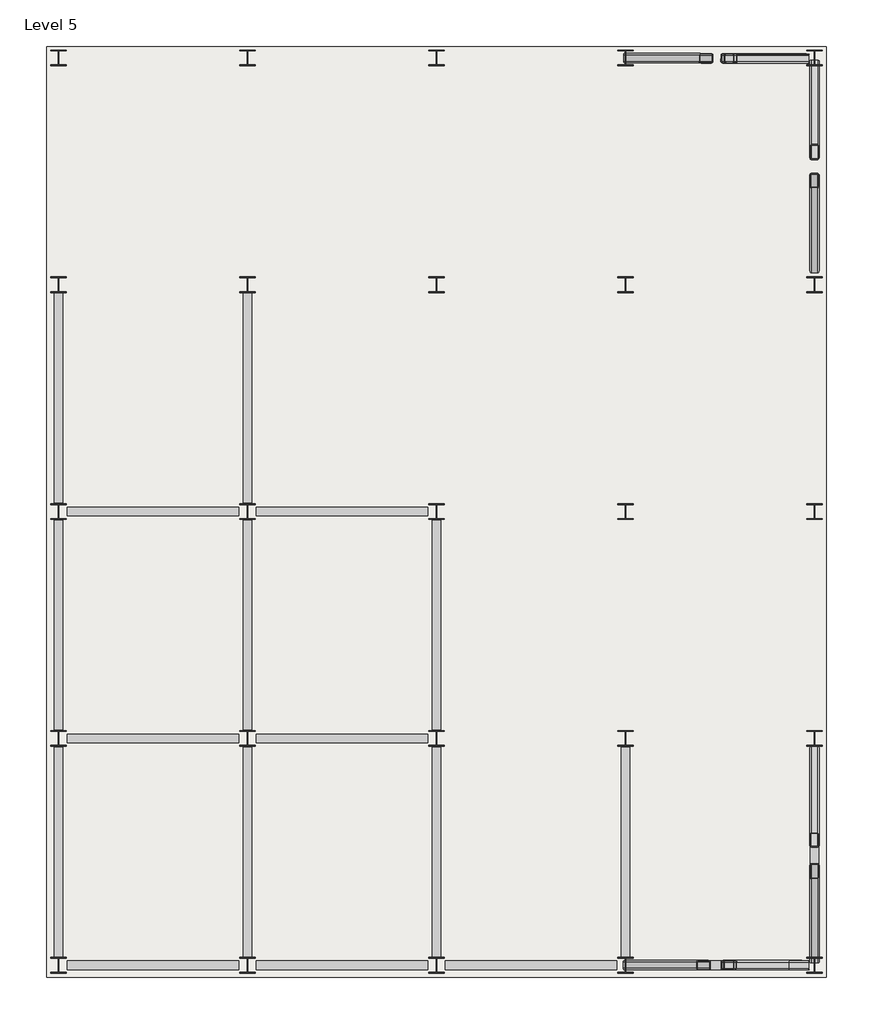
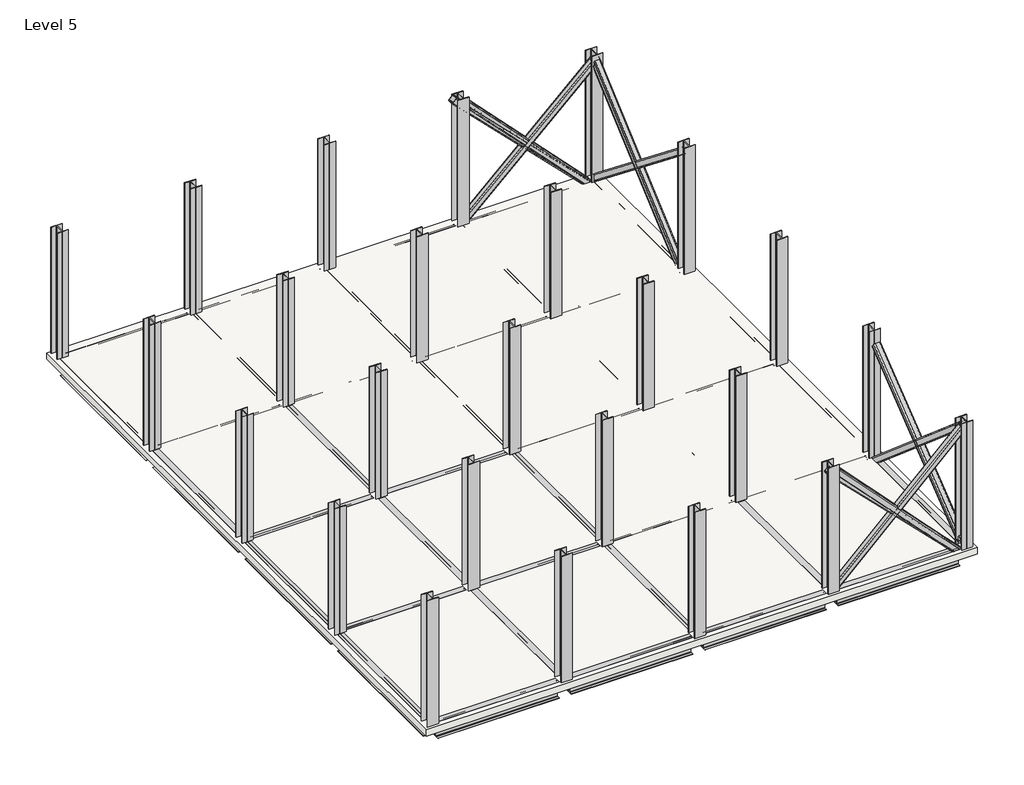
# One storey: 40 beams, 25 columns, 10 members, 1 slab.
"""IFC4 building model written with IfcOpenShell, lengths in millimetres."""

from ifc_helpers import new_model, si_unit, frame, origin, place, context, project, spatial, polyline, outline, extrude, transform, mapped, element, save
from components import w_shapes_w16x26_71b85d0e, w_shapes_w16x26_5730d789, w_shapes_column_w10x49_51893fb5, hss_square_hss6x6x1_2_008024fe, hss_square_hss6x6x1_2_53b34d95, hss_square_hss6x6x1_2_5f011b37, hss_square_hss6x6x1_2_b9926e2d, hss_square_hss6x6x1_2_d64262a5, hss_square_hss6x6x1_2_e6555cf9, hss_square_hss6x6x1_2_f7a49a43, hss_square_hss6x6x1_2_c82ee425, hss_square_hss6x6x1_2_10b7330d, hss_square_hss6x6x1_2_f3b36863

model = new_model("IFC4")

# Units and contexts
model_context = context("Model", 3, world=origin())
ifc_project = project(units=[si_unit("LENGTHUNIT", "METRE", prefix="MILLI")], contexts=[model_context])

# Site, building, storey
site = spatial("IfcSite", under=ifc_project)
building = spatial("IfcBuilding", under=site)
storey = spatial("IfcBuildingStorey", under=building, Name="Level 5", Elevation=12192.0)

# Beams
placement = place(None, origin())
w_shapes_w16x26_shape = w_shapes_w16x26_71b85d0e(model_context)
element("IfcBeam", 1, ObjectType="W Shapes : W16X26", at=placement, inside=storey, context=model_context, shape_type="MappedRepresentation", body=[
    mapped(w_shapes_w16x26_shape, transform((-5883.5186598, -2213.7239423, 11992.61), x_axis=(1.0, 0.0, 0.0), y_axis=(0.0, 1.0, 0.0), z_axis=(0.0, 0.0, 1.0))),
])
element("IfcBeam", 2, ObjectType="W Shapes : W16X26", at=placement, inside=storey, context=model_context, shape_type="MappedRepresentation", body=[
    mapped(w_shapes_w16x26_shape, transform((-2835.5186598, -2213.7239423, 11992.61), x_axis=(1.0, 0.0, 0.0), y_axis=(0.0, 1.0, 0.0), z_axis=(0.0, 0.0, 1.0))),
])
element("IfcBeam", 3, ObjectType="W Shapes : W16X26", at=placement, inside=storey, context=model_context, shape_type="MappedRepresentation", body=[
    mapped(w_shapes_w16x26_shape, transform((212.4813402, -2213.7239423, 11992.61), x_axis=(1.0, 0.0, 0.0), y_axis=(0.0, 1.0, 0.0), z_axis=(0.0, 0.0, 1.0))),
])
element("IfcBeam", 4, ObjectType="W Shapes : W16X26", at=placement, inside=storey, context=model_context, shape_type="MappedRepresentation", body=[
    mapped(w_shapes_w16x26_shape, transform((3260.4813402, -2213.7239423, 11992.61), x_axis=(1.0, 0.0, 0.0), y_axis=(0.0, 1.0, 0.0), z_axis=(0.0, 0.0, 1.0))),
])
element("IfcBeam", 5, ObjectType="W Shapes : W16X26", at=placement, inside=storey, context=model_context, shape_type="MappedRepresentation", body=[
    mapped(w_shapes_w16x26_shape, transform((-5883.5186598, 1443.8760577, 11992.61), x_axis=(1.0, 0.0, 0.0), y_axis=(0.0, 1.0, 0.0), z_axis=(0.0, 0.0, 1.0))),
])
element("IfcBeam", 6, ObjectType="W Shapes : W16X26", at=placement, inside=storey, context=model_context, shape_type="MappedRepresentation", body=[
    mapped(w_shapes_w16x26_shape, transform((-2835.5186598, 1443.8760577, 11992.61), x_axis=(1.0, 0.0, 0.0), y_axis=(0.0, 1.0, 0.0), z_axis=(0.0, 0.0, 1.0))),
])
element("IfcBeam", 7, ObjectType="W Shapes : W16X26", at=placement, inside=storey, context=model_context, shape_type="MappedRepresentation", body=[
    mapped(w_shapes_w16x26_shape, transform((212.4813402, 1443.8760577, 11992.61), x_axis=(1.0, 0.0, 0.0), y_axis=(0.0, 1.0, 0.0), z_axis=(0.0, 0.0, 1.0))),
])
element("IfcBeam", 8, ObjectType="W Shapes : W16X26", at=placement, inside=storey, context=model_context, shape_type="MappedRepresentation", body=[
    mapped(w_shapes_w16x26_shape, transform((3260.4813402, 1443.8760577, 11992.61), x_axis=(1.0, 0.0, 0.0), y_axis=(0.0, 1.0, 0.0), z_axis=(0.0, 0.0, 1.0))),
])
element("IfcBeam", 9, ObjectType="W Shapes : W16X26", at=placement, inside=storey, context=model_context, shape_type="MappedRepresentation", body=[
    mapped(w_shapes_w16x26_shape, transform((-5883.5186598, 5101.4760577, 11992.61), x_axis=(1.0, 0.0, 0.0), y_axis=(0.0, 1.0, 0.0), z_axis=(0.0, 0.0, 1.0))),
])
element("IfcBeam", 10, ObjectType="W Shapes : W16X26", at=placement, inside=storey, context=model_context, shape_type="MappedRepresentation", body=[
    mapped(w_shapes_w16x26_shape, transform((-2835.5186598, 5101.4760577, 11992.61), x_axis=(1.0, 0.0, 0.0), y_axis=(0.0, 1.0, 0.0), z_axis=(0.0, 0.0, 1.0))),
])
element("IfcBeam", 11, ObjectType="W Shapes : W16X26", at=placement, inside=storey, context=model_context, shape_type="MappedRepresentation", body=[
    mapped(w_shapes_w16x26_shape, transform((212.4813402, 5101.4760577, 11992.61), x_axis=(1.0, 0.0, 0.0), y_axis=(0.0, 1.0, 0.0), z_axis=(0.0, 0.0, 1.0))),
])
element("IfcBeam", 12, ObjectType="W Shapes : W16X26", at=placement, inside=storey, context=model_context, shape_type="MappedRepresentation", body=[
    mapped(w_shapes_w16x26_shape, transform((3260.4813402, 5101.4760577, 11992.61), x_axis=(1.0, 0.0, 0.0), y_axis=(0.0, 1.0, 0.0), z_axis=(0.0, 0.0, 1.0))),
])
element("IfcBeam", 13, ObjectType="W Shapes : W16X26", at=placement, inside=storey, context=model_context, shape_type="MappedRepresentation", body=[
    mapped(w_shapes_w16x26_shape, transform((-5883.5186598, 8759.0760577, 11992.61), x_axis=(1.0, 0.0, 0.0), y_axis=(0.0, 1.0, 0.0), z_axis=(0.0, 0.0, 1.0))),
])
element("IfcBeam", 14, ObjectType="W Shapes : W16X26", at=placement, inside=storey, context=model_context, shape_type="MappedRepresentation", body=[
    mapped(w_shapes_w16x26_shape, transform((-2835.5186598, 8759.0760577, 11992.61), x_axis=(1.0, 0.0, 0.0), y_axis=(0.0, 1.0, 0.0), z_axis=(0.0, 0.0, 1.0))),
])
element("IfcBeam", 15, ObjectType="W Shapes : W16X26", at=placement, inside=storey, context=model_context, shape_type="MappedRepresentation", body=[
    mapped(w_shapes_w16x26_shape, transform((212.4813402, 8759.0760577, 11992.61), x_axis=(1.0, 0.0, 0.0), y_axis=(0.0, 1.0, 0.0), z_axis=(0.0, 0.0, 1.0))),
])
element("IfcBeam", 16, ObjectType="W Shapes : W16X26", at=placement, inside=storey, context=model_context, shape_type="MappedRepresentation", body=[
    mapped(w_shapes_w16x26_shape, transform((3260.4813402, 8759.0760577, 11992.61), x_axis=(1.0, 0.0, 0.0), y_axis=(0.0, 1.0, 0.0), z_axis=(0.0, 0.0, 1.0))),
])
element("IfcBeam", 17, ObjectType="W Shapes : W16X26", at=placement, inside=storey, context=model_context, shape_type="MappedRepresentation", body=[
    mapped(w_shapes_w16x26_shape, transform((-5883.5186598, 12416.6760577, 11992.61), x_axis=(1.0, 0.0, 0.0), y_axis=(0.0, 1.0, 0.0), z_axis=(0.0, 0.0, 1.0))),
])
element("IfcBeam", 18, ObjectType="W Shapes : W16X26", at=placement, inside=storey, context=model_context, shape_type="MappedRepresentation", body=[
    mapped(w_shapes_w16x26_shape, transform((-2835.5186598, 12416.6760577, 11992.61), x_axis=(1.0, 0.0, 0.0), y_axis=(0.0, 1.0, 0.0), z_axis=(0.0, 0.0, 1.0))),
])
element("IfcBeam", 19, ObjectType="W Shapes : W16X26", at=placement, inside=storey, context=model_context, shape_type="MappedRepresentation", body=[
    mapped(w_shapes_w16x26_shape, transform((212.4813402, 12416.6760577, 11992.61), x_axis=(1.0, 0.0, 0.0), y_axis=(0.0, 1.0, 0.0), z_axis=(0.0, 0.0, 1.0))),
])
element("IfcBeam", 20, ObjectType="W Shapes : W16X26", at=placement, inside=storey, context=model_context, shape_type="MappedRepresentation", body=[
    mapped(w_shapes_w16x26_shape, transform((3260.4813402, 12416.6760577, 11992.61), x_axis=(1.0, 0.0, 0.0), y_axis=(0.0, 1.0, 0.0), z_axis=(0.0, 0.0, 1.0))),
])
w_shapes_w16x26_2_shape = w_shapes_w16x26_5730d789(model_context)
element("IfcBeam", 21, ObjectType="W Shapes : W16X26", at=placement, inside=storey, context=model_context, shape_type="MappedRepresentation", body=[
    mapped(w_shapes_w16x26_2_shape, transform((4784.4813402, 10587.8760577, 11992.61), x_axis=(0.0, -1.0, 0.0), y_axis=(1.0, 0.0, 0.0), z_axis=(0.0, 0.0, 1.0))),
])
element("IfcBeam", 22, ObjectType="W Shapes : W16X26", at=placement, inside=storey, context=model_context, shape_type="MappedRepresentation", body=[
    mapped(w_shapes_w16x26_2_shape, transform((4784.4813402, 6930.2760577, 11992.61), x_axis=(0.0, -1.0, 0.0), y_axis=(1.0, 0.0, 0.0), z_axis=(0.0, 0.0, 1.0))),
])
element("IfcBeam", 23, ObjectType="W Shapes : W16X26", at=placement, inside=storey, context=model_context, shape_type="MappedRepresentation", body=[
    mapped(w_shapes_w16x26_2_shape, transform((4784.4813402, 3272.6760577, 11992.61), x_axis=(0.0, -1.0, 0.0), y_axis=(1.0, 0.0, 0.0), z_axis=(0.0, 0.0, 1.0))),
])
element("IfcBeam", 24, ObjectType="W Shapes : W16X26", at=placement, inside=storey, context=model_context, shape_type="MappedRepresentation", body=[
    mapped(w_shapes_w16x26_2_shape, transform((4784.4813402, -384.9239423, 11992.61), x_axis=(0.0, -1.0, 0.0), y_axis=(1.0, 0.0, 0.0), z_axis=(0.0, 0.0, 1.0))),
])
element("IfcBeam", 25, ObjectType="W Shapes : W16X26", at=placement, inside=storey, context=model_context, shape_type="MappedRepresentation", body=[
    mapped(w_shapes_w16x26_2_shape, transform((1736.4813402, 10587.8760577, 11992.61), x_axis=(0.0, -1.0, 0.0), y_axis=(1.0, 0.0, 0.0), z_axis=(0.0, 0.0, 1.0))),
])
element("IfcBeam", 26, ObjectType="W Shapes : W16X26", at=placement, inside=storey, context=model_context, shape_type="MappedRepresentation", body=[
    mapped(w_shapes_w16x26_2_shape, transform((1736.4813402, 6930.2760577, 11992.61), x_axis=(0.0, -1.0, 0.0), y_axis=(1.0, 0.0, 0.0), z_axis=(0.0, 0.0, 1.0))),
])
element("IfcBeam", 27, ObjectType="W Shapes : W16X26", at=placement, inside=storey, context=model_context, shape_type="MappedRepresentation", body=[
    mapped(w_shapes_w16x26_2_shape, transform((1736.4813402, 3272.6760577, 11992.61), x_axis=(0.0, -1.0, 0.0), y_axis=(1.0, 0.0, 0.0), z_axis=(0.0, 0.0, 1.0))),
])
element("IfcBeam", 28, ObjectType="W Shapes : W16X26", at=placement, inside=storey, context=model_context, shape_type="MappedRepresentation", body=[
    mapped(w_shapes_w16x26_2_shape, transform((1736.4813402, -384.9239423, 11992.61), x_axis=(0.0, -1.0, 0.0), y_axis=(1.0, 0.0, 0.0), z_axis=(0.0, 0.0, 1.0))),
])
element("IfcBeam", 29, ObjectType="W Shapes : W16X26", at=placement, inside=storey, context=model_context, shape_type="MappedRepresentation", body=[
    mapped(w_shapes_w16x26_2_shape, transform((-1311.5186598, 10587.8760577, 11992.61), x_axis=(0.0, -1.0, 0.0), y_axis=(1.0, 0.0, 0.0), z_axis=(0.0, 0.0, 1.0))),
])
element("IfcBeam", 30, ObjectType="W Shapes : W16X26", at=placement, inside=storey, context=model_context, shape_type="MappedRepresentation", body=[
    mapped(w_shapes_w16x26_2_shape, transform((-1311.5186598, 6930.2760577, 11992.61), x_axis=(0.0, -1.0, 0.0), y_axis=(1.0, 0.0, 0.0), z_axis=(0.0, 0.0, 1.0))),
])
element("IfcBeam", 31, ObjectType="W Shapes : W16X26", at=placement, inside=storey, context=model_context, shape_type="MappedRepresentation", body=[
    mapped(w_shapes_w16x26_2_shape, transform((-1311.5186598, 3272.6760577, 11992.61), x_axis=(0.0, -1.0, 0.0), y_axis=(1.0, 0.0, 0.0), z_axis=(0.0, 0.0, 1.0))),
])
element("IfcBeam", 32, ObjectType="W Shapes : W16X26", at=placement, inside=storey, context=model_context, shape_type="MappedRepresentation", body=[
    mapped(w_shapes_w16x26_2_shape, transform((-1311.5186598, -384.9239423, 11992.61), x_axis=(0.0, -1.0, 0.0), y_axis=(1.0, 0.0, 0.0), z_axis=(0.0, 0.0, 1.0))),
])
element("IfcBeam", 33, ObjectType="W Shapes : W16X26", at=placement, inside=storey, context=model_context, shape_type="MappedRepresentation", body=[
    mapped(w_shapes_w16x26_2_shape, transform((-4359.5186598, 10587.8760577, 11992.61), x_axis=(0.0, -1.0, 0.0), y_axis=(1.0, 0.0, 0.0), z_axis=(0.0, 0.0, 1.0))),
])
element("IfcBeam", 34, ObjectType="W Shapes : W16X26", at=placement, inside=storey, context=model_context, shape_type="MappedRepresentation", body=[
    mapped(w_shapes_w16x26_2_shape, transform((-4359.5186598, 6930.2760577, 11992.61), x_axis=(0.0, -1.0, 0.0), y_axis=(1.0, 0.0, 0.0), z_axis=(0.0, 0.0, 1.0))),
])
element("IfcBeam", 35, ObjectType="W Shapes : W16X26", at=placement, inside=storey, context=model_context, shape_type="MappedRepresentation", body=[
    mapped(w_shapes_w16x26_2_shape, transform((-4359.5186598, 3272.6760577, 11992.61), x_axis=(0.0, -1.0, 0.0), y_axis=(1.0, 0.0, 0.0), z_axis=(0.0, 0.0, 1.0))),
])
element("IfcBeam", 36, ObjectType="W Shapes : W16X26", at=placement, inside=storey, context=model_context, shape_type="MappedRepresentation", body=[
    mapped(w_shapes_w16x26_2_shape, transform((-4359.5186598, -384.9239423, 11992.61), x_axis=(0.0, -1.0, 0.0), y_axis=(1.0, 0.0, 0.0), z_axis=(0.0, 0.0, 1.0))),
])
element("IfcBeam", 37, ObjectType="W Shapes : W16X26", at=placement, inside=storey, context=model_context, shape_type="MappedRepresentation", body=[
    mapped(w_shapes_w16x26_2_shape, transform((-7407.5186598, 10587.8760577, 11992.61), x_axis=(0.0, -1.0, 0.0), y_axis=(1.0, 0.0, 0.0), z_axis=(0.0, 0.0, 1.0))),
])
element("IfcBeam", 38, ObjectType="W Shapes : W16X26", at=placement, inside=storey, context=model_context, shape_type="MappedRepresentation", body=[
    mapped(w_shapes_w16x26_2_shape, transform((-7407.5186598, 6930.2760577, 11992.61), x_axis=(0.0, -1.0, 0.0), y_axis=(1.0, 0.0, 0.0), z_axis=(0.0, 0.0, 1.0))),
])
element("IfcBeam", 39, ObjectType="W Shapes : W16X26", at=placement, inside=storey, context=model_context, shape_type="MappedRepresentation", body=[
    mapped(w_shapes_w16x26_2_shape, transform((-7407.5186598, 3272.6760577, 11992.61), x_axis=(0.0, -1.0, 0.0), y_axis=(1.0, 0.0, 0.0), z_axis=(0.0, 0.0, 1.0))),
])
element("IfcBeam", 40, ObjectType="W Shapes : W16X26", at=placement, inside=storey, context=model_context, shape_type="MappedRepresentation", body=[
    mapped(w_shapes_w16x26_2_shape, transform((-7407.5186598, -384.9239423, 11992.61), x_axis=(0.0, -1.0, 0.0), y_axis=(1.0, 0.0, 0.0), z_axis=(0.0, 0.0, 1.0))),
])

# Columns
w_shapes_column_w10x49_shape = w_shapes_column_w10x49_51893fb5(model_context)
element("IfcColumn", 41, ObjectType="W Shapes-Column : W10X49", at=placement, inside=storey, context=model_context, shape_type="MappedRepresentation", body=[
    mapped(w_shapes_column_w10x49_shape, transform((4784.4813402, -2213.7239423, 0.0), x_axis=(1.0, 0.0, 0.0), y_axis=(0.0, 1.0, 0.0), z_axis=(0.0, 0.0, 1.0))),
])
element("IfcColumn", 42, ObjectType="W Shapes-Column : W10X49", at=placement, inside=storey, context=model_context, shape_type="MappedRepresentation", body=[
    mapped(w_shapes_column_w10x49_shape, transform((1736.4813402, -2213.7239423, 0.0), x_axis=(1.0, 0.0, 0.0), y_axis=(0.0, 1.0, 0.0), z_axis=(0.0, 0.0, 1.0))),
])
element("IfcColumn", 43, ObjectType="W Shapes-Column : W10X49", at=placement, inside=storey, context=model_context, shape_type="MappedRepresentation", body=[
    mapped(w_shapes_column_w10x49_shape, transform((-1311.5186598, -2213.7239423, 0.0), x_axis=(1.0, 0.0, 0.0), y_axis=(0.0, 1.0, 0.0), z_axis=(0.0, 0.0, 1.0))),
])
element("IfcColumn", 44, ObjectType="W Shapes-Column : W10X49", at=placement, inside=storey, context=model_context, shape_type="MappedRepresentation", body=[
    mapped(w_shapes_column_w10x49_shape, transform((-4359.5186598, -2213.7239423, 0.0), x_axis=(1.0, 0.0, 0.0), y_axis=(0.0, 1.0, 0.0), z_axis=(0.0, 0.0, 1.0))),
])
element("IfcColumn", 45, ObjectType="W Shapes-Column : W10X49", at=placement, inside=storey, context=model_context, shape_type="MappedRepresentation", body=[
    mapped(w_shapes_column_w10x49_shape, transform((-7407.5186598, -2213.7239423, 0.0), x_axis=(1.0, 0.0, 0.0), y_axis=(0.0, 1.0, 0.0), z_axis=(0.0, 0.0, 1.0))),
])
element("IfcColumn", 46, ObjectType="W Shapes-Column : W10X49", at=placement, inside=storey, context=model_context, shape_type="MappedRepresentation", body=[
    mapped(w_shapes_column_w10x49_shape, transform((4784.4813402, 1443.8760577, 0.0), x_axis=(1.0, 0.0, 0.0), y_axis=(0.0, 1.0, 0.0), z_axis=(0.0, 0.0, 1.0))),
])
element("IfcColumn", 47, ObjectType="W Shapes-Column : W10X49", at=placement, inside=storey, context=model_context, shape_type="MappedRepresentation", body=[
    mapped(w_shapes_column_w10x49_shape, transform((4784.4813402, 5101.4760577, 0.0), x_axis=(1.0, 0.0, 0.0), y_axis=(0.0, 1.0, 0.0), z_axis=(0.0, 0.0, 1.0))),
])
element("IfcColumn", 48, ObjectType="W Shapes-Column : W10X49", at=placement, inside=storey, context=model_context, shape_type="MappedRepresentation", body=[
    mapped(w_shapes_column_w10x49_shape, transform((4784.4813402, 8759.0760577, 0.0), x_axis=(1.0, 0.0, 0.0), y_axis=(0.0, 1.0, 0.0), z_axis=(0.0, 0.0, 1.0))),
])
element("IfcColumn", 49, ObjectType="W Shapes-Column : W10X49", at=placement, inside=storey, context=model_context, shape_type="MappedRepresentation", body=[
    mapped(w_shapes_column_w10x49_shape, transform((4784.4813402, 12416.6760577, 0.0), x_axis=(1.0, 0.0, 0.0), y_axis=(0.0, 1.0, 0.0), z_axis=(0.0, 0.0, 1.0))),
])
element("IfcColumn", 50, ObjectType="W Shapes-Column : W10X49", at=placement, inside=storey, context=model_context, shape_type="MappedRepresentation", body=[
    mapped(w_shapes_column_w10x49_shape, transform((1736.4813402, 1443.8760577, 0.0), x_axis=(1.0, 0.0, 0.0), y_axis=(0.0, 1.0, 0.0), z_axis=(0.0, 0.0, 1.0))),
])
element("IfcColumn", 51, ObjectType="W Shapes-Column : W10X49", at=placement, inside=storey, context=model_context, shape_type="MappedRepresentation", body=[
    mapped(w_shapes_column_w10x49_shape, transform((-1311.5186598, 1443.8760577, 0.0), x_axis=(1.0, 0.0, 0.0), y_axis=(0.0, 1.0, 0.0), z_axis=(0.0, 0.0, 1.0))),
])
element("IfcColumn", 52, ObjectType="W Shapes-Column : W10X49", at=placement, inside=storey, context=model_context, shape_type="MappedRepresentation", body=[
    mapped(w_shapes_column_w10x49_shape, transform((-4359.5186598, 1443.8760577, 0.0), x_axis=(1.0, 0.0, 0.0), y_axis=(0.0, 1.0, 0.0), z_axis=(0.0, 0.0, 1.0))),
])
element("IfcColumn", 53, ObjectType="W Shapes-Column : W10X49", at=placement, inside=storey, context=model_context, shape_type="MappedRepresentation", body=[
    mapped(w_shapes_column_w10x49_shape, transform((-7407.5186598, 1443.8760577, 0.0), x_axis=(1.0, 0.0, 0.0), y_axis=(0.0, 1.0, 0.0), z_axis=(0.0, 0.0, 1.0))),
])
element("IfcColumn", 54, ObjectType="W Shapes-Column : W10X49", at=placement, inside=storey, context=model_context, shape_type="MappedRepresentation", body=[
    mapped(w_shapes_column_w10x49_shape, transform((1736.4813402, 5101.4760577, 0.0), x_axis=(1.0, 0.0, 0.0), y_axis=(0.0, 1.0, 0.0), z_axis=(0.0, 0.0, 1.0))),
])
element("IfcColumn", 55, ObjectType="W Shapes-Column : W10X49", at=placement, inside=storey, context=model_context, shape_type="MappedRepresentation", body=[
    mapped(w_shapes_column_w10x49_shape, transform((-1311.5186598, 5101.4760577, 0.0), x_axis=(1.0, 0.0, 0.0), y_axis=(0.0, 1.0, 0.0), z_axis=(0.0, 0.0, 1.0))),
])
element("IfcColumn", 56, ObjectType="W Shapes-Column : W10X49", at=placement, inside=storey, context=model_context, shape_type="MappedRepresentation", body=[
    mapped(w_shapes_column_w10x49_shape, transform((-4359.5186598, 5101.4760577, 0.0), x_axis=(1.0, 0.0, 0.0), y_axis=(0.0, 1.0, 0.0), z_axis=(0.0, 0.0, 1.0))),
])
element("IfcColumn", 57, ObjectType="W Shapes-Column : W10X49", at=placement, inside=storey, context=model_context, shape_type="MappedRepresentation", body=[
    mapped(w_shapes_column_w10x49_shape, transform((-7407.5186598, 5101.4760577, 0.0), x_axis=(1.0, 0.0, 0.0), y_axis=(0.0, 1.0, 0.0), z_axis=(0.0, 0.0, 1.0))),
])
element("IfcColumn", 58, ObjectType="W Shapes-Column : W10X49", at=placement, inside=storey, context=model_context, shape_type="MappedRepresentation", body=[
    mapped(w_shapes_column_w10x49_shape, transform((1736.4813402, 8759.0760577, 0.0), x_axis=(1.0, 0.0, 0.0), y_axis=(0.0, 1.0, 0.0), z_axis=(0.0, 0.0, 1.0))),
])
element("IfcColumn", 59, ObjectType="W Shapes-Column : W10X49", at=placement, inside=storey, context=model_context, shape_type="MappedRepresentation", body=[
    mapped(w_shapes_column_w10x49_shape, transform((-1311.5186598, 8759.0760577, 0.0), x_axis=(1.0, 0.0, 0.0), y_axis=(0.0, 1.0, 0.0), z_axis=(0.0, 0.0, 1.0))),
])
element("IfcColumn", 60, ObjectType="W Shapes-Column : W10X49", at=placement, inside=storey, context=model_context, shape_type="MappedRepresentation", body=[
    mapped(w_shapes_column_w10x49_shape, transform((-4359.5186598, 8759.0760577, 0.0), x_axis=(1.0, 0.0, 0.0), y_axis=(0.0, 1.0, 0.0), z_axis=(0.0, 0.0, 1.0))),
])
element("IfcColumn", 61, ObjectType="W Shapes-Column : W10X49", at=placement, inside=storey, context=model_context, shape_type="MappedRepresentation", body=[
    mapped(w_shapes_column_w10x49_shape, transform((-7407.5186598, 8759.0760577, 0.0), x_axis=(1.0, 0.0, 0.0), y_axis=(0.0, 1.0, 0.0), z_axis=(0.0, 0.0, 1.0))),
])
element("IfcColumn", 62, ObjectType="W Shapes-Column : W10X49", at=placement, inside=storey, context=model_context, shape_type="MappedRepresentation", body=[
    mapped(w_shapes_column_w10x49_shape, transform((1736.4813402, 12416.6760577, 0.0), x_axis=(1.0, 0.0, 0.0), y_axis=(0.0, 1.0, 0.0), z_axis=(0.0, 0.0, 1.0))),
])
element("IfcColumn", 63, ObjectType="W Shapes-Column : W10X49", at=placement, inside=storey, context=model_context, shape_type="MappedRepresentation", body=[
    mapped(w_shapes_column_w10x49_shape, transform((-1311.5186598, 12416.6760577, 0.0), x_axis=(1.0, 0.0, 0.0), y_axis=(0.0, 1.0, 0.0), z_axis=(0.0, 0.0, 1.0))),
])
element("IfcColumn", 64, ObjectType="W Shapes-Column : W10X49", at=placement, inside=storey, context=model_context, shape_type="MappedRepresentation", body=[
    mapped(w_shapes_column_w10x49_shape, transform((-4359.5186598, 12416.6760577, 0.0), x_axis=(1.0, 0.0, 0.0), y_axis=(0.0, 1.0, 0.0), z_axis=(0.0, 0.0, 1.0))),
])
element("IfcColumn", 65, ObjectType="W Shapes-Column : W10X49", at=placement, inside=storey, context=model_context, shape_type="MappedRepresentation", body=[
    mapped(w_shapes_column_w10x49_shape, transform((-7407.5186598, 12416.6760577, 0.0), x_axis=(1.0, 0.0, 0.0), y_axis=(0.0, 1.0, 0.0), z_axis=(0.0, 0.0, 1.0))),
])

# Members
hss_square_hss6x6x1_2_shape = hss_square_hss6x6x1_2_008024fe(model_context)
element("IfcMember", 66, ObjectType="HSS Square : HSS6X6X1/2", at=placement, inside=storey, context=model_context, shape_type="MappedRepresentation", body=[
    mapped(hss_square_hss6x6x1_2_shape, transform((4784.4813402, 10587.8760577, 13639.8), x_axis=(0.0, 0.7840458244617616, -0.6207029443655613), y_axis=(-1.0000000000000002, 0.0, 0.0), z_axis=(0.0, 0.6207029443655613, 0.7840458244617616))),
])
hss_square_hss6x6x1_2_2_shape = hss_square_hss6x6x1_2_53b34d95(model_context)
element("IfcMember", 67, ObjectType="HSS Square : HSS6X6X1/2", at=placement, inside=storey, context=model_context, shape_type="MappedRepresentation", body=[
    mapped(hss_square_hss6x6x1_2_2_shape, transform((4784.4813402, 10626.583403, 13556.1631022), x_axis=(0.0, -0.7531556274501068, -0.6578423829765276), y_axis=(1.0000000000000002, 0.0, 0.0), z_axis=(0.0, -0.6578423829765276, 0.7531556274501068))),
])
hss_square_hss6x6x1_2_3_shape = hss_square_hss6x6x1_2_5f011b37(model_context)
element("IfcMember", 68, ObjectType="HSS Square : HSS6X6X1/2", at=placement, inside=storey, context=model_context, shape_type="MappedRepresentation", body=[
    mapped(hss_square_hss6x6x1_2_3_shape, transform((4784.4813402, -384.9239423, 13556.1631022), x_axis=(0.0, 0.7600753460328191, -0.6498349547024158), y_axis=(-1.0000000000000002, 0.0, 0.0), z_axis=(0.0, 0.6498349547024158, 0.7600753460328191))),
])
hss_square_hss6x6x1_2_4_shape = hss_square_hss6x6x1_2_b9926e2d(model_context)
element("IfcMember", 69, ObjectType="HSS Square : HSS6X6X1/2", at=placement, inside=storey, context=model_context, shape_type="MappedRepresentation", body=[
    mapped(hss_square_hss6x6x1_2_4_shape, transform((4784.4813402, -384.9239423, 13639.8), x_axis=(0.0, -0.7840458244617616, -0.6207029443655613), y_axis=(1.0000000000000002, 0.0, 0.0), z_axis=(0.0, -0.6207029443655613, 0.7840458244617616))),
])
hss_square_hss6x6x1_2_5_shape = hss_square_hss6x6x1_2_d64262a5(model_context)
element("IfcMember", 70, ObjectType="HSS Square : HSS6X6X1/2", at=placement, inside=storey, context=model_context, shape_type="MappedRepresentation", body=[
    mapped(hss_square_hss6x6x1_2_5_shape, transform((3306.3591493, -2213.7239423, 13516.61), x_axis=(0.6910908469701543, 0.0, -0.7227679027420042), y_axis=(0.0, 1.0000000000000002, 0.0), z_axis=(0.7227679027420042, 0.0, 0.6910908469701543))),
])
hss_square_hss6x6x1_2_6_shape = hss_square_hss6x6x1_2_e6555cf9(model_context)
element("IfcMember", 71, ObjectType="HSS Square : HSS6X6X1/2", at=placement, inside=storey, context=model_context, shape_type="MappedRepresentation", body=[
    mapped(hss_square_hss6x6x1_2_6_shape, transform((3168.0352384, -2213.7239423, 13557.8521986), x_axis=(-0.718393447364439, 0.0, -0.6956370136672122), y_axis=(0.0, -1.0000000000000002, 0.0), z_axis=(-0.6956370136672122, 0.0, 0.718393447364439))),
])
hss_square_hss6x6x1_2_7_shape = hss_square_hss6x6x1_2_f7a49a43(model_context)
element("IfcMember", 72, ObjectType="HSS Square : HSS6X6X1/2", at=placement, inside=storey, context=model_context, shape_type="MappedRepresentation", body=[
    mapped(hss_square_hss6x6x1_2_7_shape, transform((3260.4813402, -2213.7239423, 13516.61), x_axis=(0.7071067811865476, 0.0, -0.7071067811865477), y_axis=(0.0, 1.0000000000000002, 0.0), z_axis=(0.7071067811865477, 0.0, 0.7071067811865476))),
])
hss_square_hss6x6x1_2_8_shape = hss_square_hss6x6x1_2_c82ee425(model_context)
element("IfcMember", 73, ObjectType="HSS Square : HSS6X6X1/2", at=placement, inside=storey, context=model_context, shape_type="MappedRepresentation", body=[
    mapped(hss_square_hss6x6x1_2_8_shape, transform((3316.8167423, 12409.9819642, 13516.61), x_axis=(0.6936649554232432, -0.003163841464712012, -0.7202908577268327), y_axis=(0.004561003884502068, 0.9999895985676881, 0.0), z_axis=(0.720283365670231, -0.0032852494000626354, 0.6936721706073726))),
])
hss_square_hss6x6x1_2_9_shape = hss_square_hss6x6x1_2_10b7330d(model_context)
element("IfcMember", 74, ObjectType="HSS Square : HSS6X6X1/2", at=placement, inside=storey, context=model_context, shape_type="MappedRepresentation", body=[
    mapped(hss_square_hss6x6x1_2_9_shape, transform((3168.0352384, 12409.9819642, 13516.61), x_axis=(-0.7276035720332942, 0.003013182054487384, -0.6859912264003803), y_axis=(-0.004141205915939179, -0.9999914251700173, 0.0), z_axis=(-0.6859853441422442, 0.002840830925050775, 0.7276098111637188))),
])
hss_square_hss6x6x1_2_10_shape = hss_square_hss6x6x1_2_f3b36863(model_context)
element("IfcMember", 75, ObjectType="HSS Square : HSS6X6X1/2", at=placement, inside=storey, context=model_context, shape_type="MappedRepresentation", body=[
    mapped(hss_square_hss6x6x1_2_10_shape, transform((3260.4813402, 12409.9819642, 13516.61), x_axis=(0.7071033705496141, -0.0031059160887349857, -0.7071033705496143), y_axis=(0.004392407470180804, 0.9999903533317791, 0.0), z_axis=(0.7070965493580005, -0.003105886126991346, 0.7071101918070303))),
])

# Slab
element("IfcSlab", 76, ObjectType="6\" Foundation Slab", at=placement, inside=storey, context=model_context, shape_type="SweptSolid", body=[
    extrude(outline(polyline([(4974.3230176, 12600.4819642), (4974.3230176, -2410.9180358), (-7598.6769824, -2410.9180358), (-7598.6769824, 12600.4819642), (4974.3230176, 12600.4819642)])), frame((0.0, 0.0, 12039.6), z_axis=(0.0, 0.0, 1.0), x_axis=(1.0, 0.0, 0.0)), (0.0, 0.0, 1.0), 152.4),
])

save(model, "model.ifc")

# Revit data of these elements
# Type "W Shapes : W16X26"
#   Section Name Key = "W16x26"
#   Assembly Code = "B10"
#   Width = 5.500"
#   Web Thickness = 0.250"
#   Web Fillet = 0.402"
#   Warping Constant = 565.00 in⁶
#   Torsional Moment of Inertia = 0.262 in⁴
#   Section Area = 7.68 in²
#   Plastic Modulus weak axis = 5.48 in³
#   Plastic Modulus strong axis = 44.20 in³
#   Perimeter = 52.20 ft²/ft
#   Nominal Weight = 26.00 lbf/ft
#   Moment of Inertia weak axis = 9.59 in⁴
#   Moment of Inertia strong axis = 301.00 in⁴
#   Height = 15.700"
#   Flange Thickness = 0.345"
#   Elastic Modulus weak axis = 3.49 in³
#   Elastic Modulus strong axis = 38.40 in³
#   Centroid Vertical = 7.850"
#   Centroid Horizontal = 2.750"
#   Bolt Spacing = 0' - 3 1/2"
#   Length [instance default] = 5' - 0"
#   Structural Material [instance default] = Steel ASTM A992
#   Principal Axes Angle = 0
# Type "W Shapes-Column : W10X49"
#   Section Name Key = "W10x49"
#   Assembly Code = "B10"
#   Width = 10.000"
#   Web Thickness = 0.340"
#   Web Fillet = 0.500"
#   Warping Constant = 2070.00 in⁶
#   Torsional Moment of Inertia = 1.39 in⁴
#   Section Area = 14.40 in²
#   Plastic Modulus weak axis = 28.30 in³
#   Plastic Modulus strong axis = 60.40 in³
#   Perimeter = 58.50 ft²/ft
#   Nominal Weight = 49.00 lbf/ft
#   Moment of Inertia weak axis = 93.40 in⁴
#   Moment of Inertia strong axis = 272.00 in⁴
#   Height = 10.000"
#   Flange Thickness = 0.560"
#   Elastic Modulus weak axis = 18.70 in³
#   Elastic Modulus strong axis = 54.60 in³
#   Centroid Vertical = 5.000"
#   Centroid Horizontal = 5.000"
#   Bolt Spacing = 0' - 5 1/2"
#   Structural Material [instance default] = Steel ASTM A992
#   Principal Axes Angle = 0
# Type "HSS Square : HSS6X6X1/2"
#   Section Name Key = "HSS 6X6X1/2"
#   Assembly Code = "B10"
#   Width = 6.000"
#   Wall Nominal Thickness = 0.500"
#   Wall Design Thickness = 0.465"
#   Torsional Moment of Inertia = 81.10 in⁴
#   Torsional Modulus = 28.10 in³
#   Section Area = 9.74 in²
#   Plastic Modulus weak axis = 19.80 in³
#   Plastic Modulus strong axis = 19.80 in³
#   Outer Fillet = 1.000"
#   Nominal Weight = 35.24 lbf/ft
#   Moment of Inertia weak axis = 48.30 in⁴
#   Moment of Inertia strong axis = 48.30 in⁴
#   Inner Fillet = 0.500"
#   Height = 6.000"
#   Elastic Modulus weak axis = 16.10 in³
#   Elastic Modulus strong axis = 16.10 in³
#   Centroid Vertical = 3.000"
#   Centroid Horizontal = 3.000"
#   Length [instance default] = 5' - 0"
#   Structural Material [instance default] = Steel ASTM A500, Grade B, Rectangular and Square
#   Principal Axes Angle = 0
# Type "6\" Foundation Slab"
#   Layers, outside or top first: 0' - 6" "Concrete, Cast-in-Place gray" (function 1)
# Elements 1, 2, 3, 4, 5, 6, 7, 8, 9, 10, 11, 12, 13, 14, 15, 16, 17, 18, 19, 20, 21, 22, 23, 24, 25, 26, 27, 28, 29, 30, 31, 32, 33, 34, 35, 36, 37, 38, 39, 40 (IfcBeam, "W Shapes : W16X26")
#   Comments = ""
#   Structural Material = Steel ASTM A992
#   Phase Created = New Construction
#   Materials on its faces: "Steel ASTM A992"
# Elements 41, 42, 43, 44, 45, 46, 47, 48, 49, 50, 51, 52, 53, 54, 55, 56, 57, 58, 59, 60, 61, 62, 63, 64, 65 (IfcColumn, "W Shapes-Column : W10X49")
#   Structural Material = Steel ASTM A992
#   Phase Created = New Construction
#   Materials on its faces: "Steel ASTM A992"
# Elements 66, 67, 68, 69, 70, 71, 72, 73, 74, 75 (IfcMember, "HSS Square : HSS6X6X1/2")
#   Comments = ""
#   Structural Material = Steel ASTM A992
#   Phase Created = New Construction
#   Materials on its faces: "Steel ASTM A992"
# Element 76 (IfcSlab, "6\" Foundation Slab")
#   Height Offset From Level = 0' - 0"
#   built-in parameter 1001954 = 1
#   Phase Created = New Construction
#   Materials on its faces: "Concrete, Cast-in-Place gray"
# Materials
#   "Steel ASTM A992": class "Metal", colour RGB 199 199 199, transparency 0, Description = "Structural steel 50ksi", Cost = 0
#   "Steel ASTM A500, Grade B, Rectangular and Square": class "Metal", colour RGB 199 199 199, transparency 0, Description = "Carbon steel", Cost = 0
#   "Concrete, Cast-in-Place gray": class "Concrete", colour RGB 192 192 192, transparency 0, Description = "Cast-in-place concrete", Cost = 0
